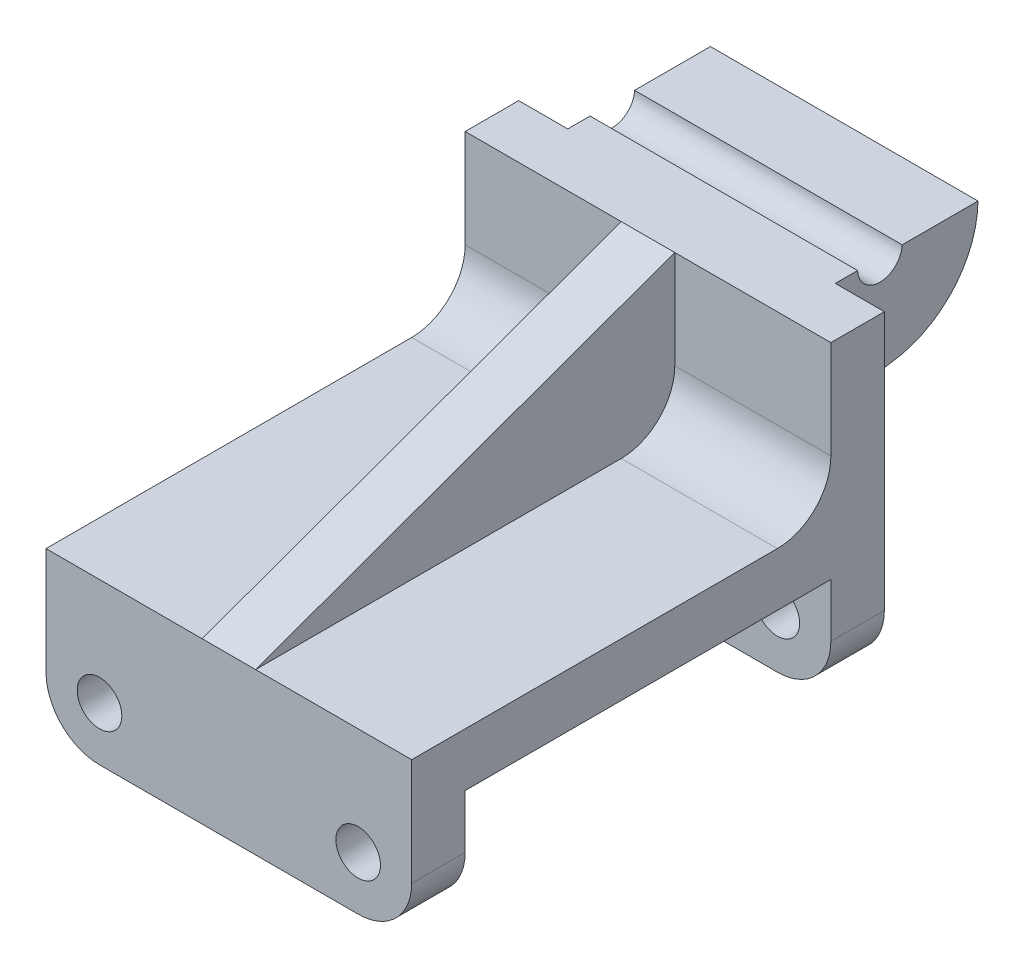
ISO-10303-21;
HEADER;
FILE_DESCRIPTION(('STEP AP214'),'2;1');
FILE_NAME('part.step','',(''),(''),'','','');
FILE_SCHEMA(('AUTOMOTIVE_DESIGN { 1 0 10303 214 1 1 1 1 }'));
ENDSEC;
DATA;
#1=APPLICATION_CONTEXT('core data for automotive mechanical design processes');
#2=APPLICATION_PROTOCOL_DEFINITION('international standard','automotive_design',2000,#1);
#3=PRODUCT_CONTEXT('',#1,'mechanical');
#4=PRODUCT('Part','Part','',(#3));
#5=PRODUCT_RELATED_PRODUCT_CATEGORY('part','',(#4));
#6=PRODUCT_DEFINITION_FORMATION('','',#4);
#7=PRODUCT_DEFINITION_CONTEXT('part definition',#1,'design');
#8=PRODUCT_DEFINITION('design','',#6,#7);
#9=PRODUCT_DEFINITION_SHAPE('','',#8);
#10=(LENGTH_UNIT() NAMED_UNIT(*) SI_UNIT(.MILLI.,.METRE.));
#11=(NAMED_UNIT(*) PLANE_ANGLE_UNIT() SI_UNIT($,.RADIAN.));
#12=(NAMED_UNIT(*) SI_UNIT($,.STERADIAN.) SOLID_ANGLE_UNIT());
#13=UNCERTAINTY_MEASURE_WITH_UNIT(LENGTH_MEASURE(1.E-05),#10,'distance_accuracy_value','');
#14=(GEOMETRIC_REPRESENTATION_CONTEXT(3) GLOBAL_UNCERTAINTY_ASSIGNED_CONTEXT((#13)) GLOBAL_UNIT_ASSIGNED_CONTEXT((#10,
#11,#12)) REPRESENTATION_CONTEXT('',''));
#15=CARTESIAN_POINT('',(0.,0.,0.));
#16=DIRECTION('',(0.,0.,1.));
#17=DIRECTION('',(1.,0.,0.));
#18=AXIS2_PLACEMENT_3D('',#15,#16,#17);
#19=CARTESIAN_POINT('',(82.,70.,-94.));
#20=DIRECTION('',(0.,0.,-1.));
#21=DIRECTION('',(-1.,0.,0.));
#22=AXIS2_PLACEMENT_3D('',#19,#20,#21);
#23=PLANE('',#22);
#24=DIRECTION('',(0.,-1.,0.));
#25=VECTOR('',#24,1.);
#26=CARTESIAN_POINT('',(0.,70.,-94.));
#27=LINE('',#26,#25);
#28=CARTESIAN_POINT('',(0.,70.,-94.));
#29=VERTEX_POINT('',#28);
#30=CARTESIAN_POINT('',(0.,48.,-94.));
#31=VERTEX_POINT('',#30);
#32=EDGE_CURVE('E315',#29,#31,#27,.T.);
#33=ORIENTED_EDGE('',*,*,#32,.T.);
#34=DIRECTION('',(-1.,0.,0.));
#35=VECTOR('',#34,1.);
#36=CARTESIAN_POINT('',(35.,48.,-94.));
#37=LINE('',#36,#35);
#38=CARTESIAN_POINT('',(35.,48.,-94.));
#39=VERTEX_POINT('',#38);
#40=EDGE_CURVE('E298',#31,#39,#37,.F.);
#41=ORIENTED_EDGE('',*,*,#40,.T.);
#42=DIRECTION('',(0.,-1.,0.));
#43=VECTOR('',#42,1.);
#44=CARTESIAN_POINT('',(35.,70.,-94.));
#45=LINE('',#44,#43);
#46=CARTESIAN_POINT('',(35.,70.,-94.));
#47=VERTEX_POINT('',#46);
#48=EDGE_CURVE('E335',#47,#39,#45,.T.);
#49=ORIENTED_EDGE('',*,*,#48,.F.);
#50=DIRECTION('',(-1.,0.,0.));
#51=VECTOR('',#50,1.);
#52=CARTESIAN_POINT('',(82.,70.,-94.));
#53=LINE('',#52,#51);
#54=EDGE_CURVE('E321',#47,#29,#53,.T.);
#55=ORIENTED_EDGE('',*,*,#54,.T.);
#56=EDGE_LOOP('',(#33,#41,#49,#55));
#57=FACE_BOUND('',#56,.T.);
#58=ADVANCED_FACE('F39',(#57),#23,.F.);
#59=CARTESIAN_POINT('',(82.,36.,-94.));
#60=DIRECTION('',(0.,-1.,0.));
#61=DIRECTION('',(0.,0.,-1.));
#62=AXIS2_PLACEMENT_3D('',#59,#60,#61);
#63=PLANE('',#62);
#64=DIRECTION('',(0.,0.,1.));
#65=VECTOR('',#64,1.);
#66=CARTESIAN_POINT('',(35.,36.,-94.));
#67=LINE('',#66,#65);
#68=CARTESIAN_POINT('',(35.,36.,-82.));
#69=VERTEX_POINT('',#68);
#70=CARTESIAN_POINT('',(35.,36.,0.));
#71=VERTEX_POINT('',#70);
#72=EDGE_CURVE('E289',#69,#71,#67,.T.);
#73=ORIENTED_EDGE('',*,*,#72,.F.);
#74=DIRECTION('',(-1.,0.,0.));
#75=VECTOR('',#74,1.);
#76=CARTESIAN_POINT('',(0.,36.,-82.));
#77=LINE('',#76,#75);
#78=CARTESIAN_POINT('',(0.,36.,-82.));
#79=VERTEX_POINT('',#78);
#80=EDGE_CURVE('E291',#69,#79,#77,.T.);
#81=ORIENTED_EDGE('',*,*,#80,.T.);
#82=DIRECTION('',(0.,0.,1.));
#83=VECTOR('',#82,1.);
#84=CARTESIAN_POINT('',(0.,36.,-94.));
#85=LINE('',#84,#83);
#86=CARTESIAN_POINT('',(0.,36.,0.));
#87=VERTEX_POINT('',#86);
#88=EDGE_CURVE('E314',#79,#87,#85,.T.);
#89=ORIENTED_EDGE('',*,*,#88,.T.);
#90=DIRECTION('',(-1.,0.,0.));
#91=VECTOR('',#90,1.);
#92=CARTESIAN_POINT('',(82.,36.,0.));
#93=LINE('',#92,#91);
#94=EDGE_CURVE('E340',#71,#87,#93,.T.);
#95=ORIENTED_EDGE('',*,*,#94,.F.);
#96=EDGE_LOOP('',(#73,#81,#89,#95));
#97=FACE_BOUND('',#96,.T.);
#98=ADVANCED_FACE('F333',(#97),#63,.F.);
#99=CARTESIAN_POINT('',(82.,36.,0.));
#100=DIRECTION('',(0.,0.,-1.));
#101=DIRECTION('',(0.,1.,0.));
#102=AXIS2_PLACEMENT_3D('',#99,#100,#101);
#103=PLANE('',#102);
#104=CARTESIAN_POINT('',(70.,12.,0.));
#105=DIRECTION('',(0.,0.,1.));
#106=DIRECTION('',(1.,0.,0.));
#107=AXIS2_PLACEMENT_3D('',#104,#105,#106);
#108=CIRCLE('',#107,5.);
#109=CARTESIAN_POINT('',(75.,12.,0.));
#110=VERTEX_POINT('',#109);
#111=EDGE_CURVE('E362',#110,#110,#108,.T.);
#112=ORIENTED_EDGE('',*,*,#111,.F.);
#113=EDGE_LOOP('',(#112));
#114=FACE_BOUND('',#113,.T.);
#115=CARTESIAN_POINT('',(82.,36.,0.));
#116=VERTEX_POINT('',#115);
#117=CARTESIAN_POINT('',(47.,36.,0.));
#118=VERTEX_POINT('',#117);
#119=EDGE_CURVE('E343',#116,#118,#93,.T.);
#120=ORIENTED_EDGE('',*,*,#119,.T.);
#121=EDGE_CURVE('E342',#118,#71,#93,.T.);
#122=ORIENTED_EDGE('',*,*,#121,.T.);
#123=ORIENTED_EDGE('',*,*,#94,.T.);
#124=DIRECTION('',(0.,-1.,0.));
#125=VECTOR('',#124,1.);
#126=CARTESIAN_POINT('',(0.,36.,0.));
#127=LINE('',#126,#125);
#128=CARTESIAN_POINT('',(0.,12.,0.));
#129=VERTEX_POINT('',#128);
#130=EDGE_CURVE('E387',#87,#129,#127,.T.);
#131=ORIENTED_EDGE('',*,*,#130,.T.);
#132=CARTESIAN_POINT('',(12.,12.,0.));
#133=DIRECTION('',(0.,0.,-1.));
#134=DIRECTION('',(0.,1.,0.));
#135=AXIS2_PLACEMENT_3D('',#132,#133,#134);
#136=CIRCLE('',#135,12.);
#137=CARTESIAN_POINT('',(12.,0.,0.));
#138=VERTEX_POINT('',#137);
#139=EDGE_CURVE('E287',#129,#138,#136,.F.);
#140=ORIENTED_EDGE('',*,*,#139,.T.);
#141=DIRECTION('',(-1.,0.,0.));
#142=VECTOR('',#141,1.);
#143=CARTESIAN_POINT('',(82.,0.,0.));
#144=LINE('',#143,#142);
#145=CARTESIAN_POINT('',(70.,0.,0.));
#146=VERTEX_POINT('',#145);
#147=EDGE_CURVE('E249',#146,#138,#144,.T.);
#148=ORIENTED_EDGE('',*,*,#147,.F.);
#149=CARTESIAN_POINT('',(70.,12.,0.));
#150=DIRECTION('',(0.,0.,-1.));
#151=DIRECTION('',(0.,1.,0.));
#152=AXIS2_PLACEMENT_3D('',#149,#150,#151);
#153=CIRCLE('',#152,12.);
#154=CARTESIAN_POINT('',(82.,12.,0.));
#155=VERTEX_POINT('',#154);
#156=EDGE_CURVE('E284',#146,#155,#153,.F.);
#157=ORIENTED_EDGE('',*,*,#156,.T.);
#158=DIRECTION('',(0.,-1.,0.));
#159=VECTOR('',#158,1.);
#160=CARTESIAN_POINT('',(82.,36.,0.));
#161=LINE('',#160,#159);
#162=EDGE_CURVE('E390',#116,#155,#161,.T.);
#163=ORIENTED_EDGE('',*,*,#162,.F.);
#164=EDGE_LOOP('',(#120,#122,#123,#131,#140,#148,#157,#163));
#165=FACE_BOUND('',#164,.T.);
#166=CARTESIAN_POINT('',(12.,12.,0.));
#167=DIRECTION('',(0.,0.,1.));
#168=DIRECTION('',(1.,0.,0.));
#169=AXIS2_PLACEMENT_3D('',#166,#167,#168);
#170=CIRCLE('',#169,5.);
#171=CARTESIAN_POINT('',(17.,12.,0.));
#172=VERTEX_POINT('',#171);
#173=EDGE_CURVE('E370',#172,#172,#170,.T.);
#174=ORIENTED_EDGE('',*,*,#173,.F.);
#175=EDGE_LOOP('',(#174));
#176=FACE_BOUND('',#175,.T.);
#177=ADVANCED_FACE('F419',(#114,#165,#176),#103,.F.);
#178=CARTESIAN_POINT('',(82.,0.,0.));
#179=DIRECTION('',(0.,1.,0.));
#180=DIRECTION('',(0.,0.,1.));
#181=AXIS2_PLACEMENT_3D('',#178,#179,#180);
#182=PLANE('',#181);
#183=ORIENTED_EDGE('',*,*,#147,.T.);
#184=DIRECTION('',(0.,0.,-1.));
#185=VECTOR('',#184,1.);
#186=CARTESIAN_POINT('',(12.,0.,0.));
#187=LINE('',#186,#185);
#188=CARTESIAN_POINT('',(12.,0.,-12.));
#189=VERTEX_POINT('',#188);
#190=EDGE_CURVE('E280',#138,#189,#187,.T.);
#191=ORIENTED_EDGE('',*,*,#190,.T.);
#192=DIRECTION('',(-1.,0.,0.));
#193=VECTOR('',#192,1.);
#194=CARTESIAN_POINT('',(82.,0.,-12.));
#195=LINE('',#194,#193);
#196=CARTESIAN_POINT('',(70.,0.,-12.));
#197=VERTEX_POINT('',#196);
#198=EDGE_CURVE('E250',#197,#189,#195,.T.);
#199=ORIENTED_EDGE('',*,*,#198,.F.);
#200=DIRECTION('',(0.,0.,-1.));
#201=VECTOR('',#200,1.);
#202=CARTESIAN_POINT('',(70.,0.,0.));
#203=LINE('',#202,#201);
#204=EDGE_CURVE('E274',#197,#146,#203,.F.);
#205=ORIENTED_EDGE('',*,*,#204,.T.);
#206=EDGE_LOOP('',(#183,#191,#199,#205));
#207=FACE_BOUND('',#206,.T.);
#208=ADVANCED_FACE('F421',(#207),#182,.F.);
#209=CARTESIAN_POINT('',(82.,0.,-12.));
#210=DIRECTION('',(0.,0.,1.));
#211=DIRECTION('',(0.,-1.,0.));
#212=AXIS2_PLACEMENT_3D('',#209,#210,#211);
#213=PLANE('',#212);
#214=CARTESIAN_POINT('',(70.,12.,-12.));
#215=DIRECTION('',(0.,0.,1.));
#216=DIRECTION('',(0.,-1.,0.));
#217=AXIS2_PLACEMENT_3D('',#214,#215,#216);
#218=CIRCLE('',#217,5.);
#219=CARTESIAN_POINT('',(70.,7.,-12.));
#220=VERTEX_POINT('',#219);
#221=EDGE_CURVE('E380',#220,#220,#218,.T.);
#222=ORIENTED_EDGE('',*,*,#221,.T.);
#223=EDGE_LOOP('',(#222));
#224=FACE_BOUND('',#223,.T.);
#225=ORIENTED_EDGE('',*,*,#198,.T.);
#226=CARTESIAN_POINT('',(12.,12.,-12.));
#227=DIRECTION('',(0.,0.,1.));
#228=DIRECTION('',(0.,-1.,0.));
#229=AXIS2_PLACEMENT_3D('',#226,#227,#228);
#230=CIRCLE('',#229,12.);
#231=CARTESIAN_POINT('',(0.,12.,-12.));
#232=VERTEX_POINT('',#231);
#233=EDGE_CURVE('E285',#189,#232,#230,.F.);
#234=ORIENTED_EDGE('',*,*,#233,.T.);
#235=DIRECTION('',(0.,1.,0.));
#236=VECTOR('',#235,1.);
#237=CARTESIAN_POINT('',(0.,0.,-12.));
#238=LINE('',#237,#236);
#239=CARTESIAN_POINT('',(0.,24.,-12.));
#240=VERTEX_POINT('',#239);
#241=EDGE_CURVE('E404',#232,#240,#238,.T.);
#242=ORIENTED_EDGE('',*,*,#241,.T.);
#243=DIRECTION('',(-1.,0.,0.));
#244=VECTOR('',#243,1.);
#245=CARTESIAN_POINT('',(82.,24.,-12.));
#246=LINE('',#245,#244);
#247=CARTESIAN_POINT('',(82.,24.,-12.));
#248=VERTEX_POINT('',#247);
#249=EDGE_CURVE('E242',#248,#240,#246,.T.);
#250=ORIENTED_EDGE('',*,*,#249,.F.);
#251=DIRECTION('',(0.,1.,0.));
#252=VECTOR('',#251,1.);
#253=CARTESIAN_POINT('',(82.,0.,-12.));
#254=LINE('',#253,#252);
#255=CARTESIAN_POINT('',(82.,12.,-12.));
#256=VERTEX_POINT('',#255);
#257=EDGE_CURVE('E388',#256,#248,#254,.T.);
#258=ORIENTED_EDGE('',*,*,#257,.F.);
#259=CARTESIAN_POINT('',(70.,12.,-12.));
#260=DIRECTION('',(0.,0.,1.));
#261=DIRECTION('',(0.,-1.,0.));
#262=AXIS2_PLACEMENT_3D('',#259,#260,#261);
#263=CIRCLE('',#262,12.);
#264=EDGE_CURVE('E278',#256,#197,#263,.F.);
#265=ORIENTED_EDGE('',*,*,#264,.T.);
#266=EDGE_LOOP('',(#225,#234,#242,#250,#258,#265));
#267=FACE_BOUND('',#266,.T.);
#268=CARTESIAN_POINT('',(12.,12.,-12.));
#269=DIRECTION('',(0.,0.,1.));
#270=DIRECTION('',(0.,-1.,0.));
#271=AXIS2_PLACEMENT_3D('',#268,#269,#270);
#272=CIRCLE('',#271,5.);
#273=CARTESIAN_POINT('',(12.,7.,-12.));
#274=VERTEX_POINT('',#273);
#275=EDGE_CURVE('E382',#274,#274,#272,.T.);
#276=ORIENTED_EDGE('',*,*,#275,.T.);
#277=EDGE_LOOP('',(#276));
#278=FACE_BOUND('',#277,.T.);
#279=ADVANCED_FACE('F436',(#224,#267,#278),#213,.F.);
#280=CARTESIAN_POINT('',(82.,24.,-12.));
#281=DIRECTION('',(0.,1.,0.));
#282=DIRECTION('',(0.,0.,1.));
#283=AXIS2_PLACEMENT_3D('',#280,#281,#282);
#284=PLANE('',#283);
#285=ORIENTED_EDGE('',*,*,#249,.T.);
#286=DIRECTION('',(0.,0.,-1.));
#287=VECTOR('',#286,1.);
#288=CARTESIAN_POINT('',(0.,24.,-12.));
#289=LINE('',#288,#287);
#290=CARTESIAN_POINT('',(0.,24.,-94.));
#291=VERTEX_POINT('',#290);
#292=EDGE_CURVE('E410',#240,#291,#289,.T.);
#293=ORIENTED_EDGE('',*,*,#292,.T.);
#294=DIRECTION('',(-1.,0.,0.));
#295=VECTOR('',#294,1.);
#296=CARTESIAN_POINT('',(82.,24.,-94.));
#297=LINE('',#296,#295);
#298=CARTESIAN_POINT('',(82.,24.,-94.));
#299=VERTEX_POINT('',#298);
#300=EDGE_CURVE('E241',#299,#291,#297,.T.);
#301=ORIENTED_EDGE('',*,*,#300,.F.);
#302=DIRECTION('',(0.,0.,-1.));
#303=VECTOR('',#302,1.);
#304=CARTESIAN_POINT('',(82.,24.,-12.));
#305=LINE('',#304,#303);
#306=EDGE_CURVE('E395',#248,#299,#305,.T.);
#307=ORIENTED_EDGE('',*,*,#306,.F.);
#308=EDGE_LOOP('',(#285,#293,#301,#307));
#309=FACE_BOUND('',#308,.T.);
#310=ADVANCED_FACE('F437',(#309),#284,.F.);
#311=CARTESIAN_POINT('',(82.,24.,-94.));
#312=DIRECTION('',(0.,0.,-1.));
#313=DIRECTION('',(0.,1.,0.));
#314=AXIS2_PLACEMENT_3D('',#311,#312,#313);
#315=PLANE('',#314);
#316=CARTESIAN_POINT('',(70.,12.,-94.));
#317=DIRECTION('',(0.,0.,-1.));
#318=DIRECTION('',(0.,1.,0.));
#319=AXIS2_PLACEMENT_3D('',#316,#317,#318);
#320=CIRCLE('',#319,5.);
#321=CARTESIAN_POINT('',(70.,17.,-94.));
#322=VERTEX_POINT('',#321);
#323=EDGE_CURVE('E368',#322,#322,#320,.T.);
#324=ORIENTED_EDGE('',*,*,#323,.T.);
#325=EDGE_LOOP('',(#324));
#326=FACE_BOUND('',#325,.T.);
#327=ORIENTED_EDGE('',*,*,#300,.T.);
#328=DIRECTION('',(0.,-1.,0.));
#329=VECTOR('',#328,1.);
#330=CARTESIAN_POINT('',(0.,24.,-94.));
#331=LINE('',#330,#329);
#332=CARTESIAN_POINT('',(0.,12.,-94.));
#333=VERTEX_POINT('',#332);
#334=EDGE_CURVE('E407',#291,#333,#331,.T.);
#335=ORIENTED_EDGE('',*,*,#334,.T.);
#336=CARTESIAN_POINT('',(12.,12.,-94.));
#337=DIRECTION('',(0.,0.,-1.));
#338=DIRECTION('',(0.,1.,0.));
#339=AXIS2_PLACEMENT_3D('',#336,#337,#338);
#340=CIRCLE('',#339,12.);
#341=CARTESIAN_POINT('',(12.,0.,-94.));
#342=VERTEX_POINT('',#341);
#343=EDGE_CURVE('E266',#333,#342,#340,.F.);
#344=ORIENTED_EDGE('',*,*,#343,.T.);
#345=DIRECTION('',(-1.,0.,0.));
#346=VECTOR('',#345,1.);
#347=CARTESIAN_POINT('',(82.,0.,-94.));
#348=LINE('',#347,#346);
#349=CARTESIAN_POINT('',(70.,0.,-94.));
#350=VERTEX_POINT('',#349);
#351=EDGE_CURVE('E237',#350,#342,#348,.T.);
#352=ORIENTED_EDGE('',*,*,#351,.F.);
#353=CARTESIAN_POINT('',(70.,12.,-94.));
#354=DIRECTION('',(0.,0.,-1.));
#355=DIRECTION('',(0.,1.,0.));
#356=AXIS2_PLACEMENT_3D('',#353,#354,#355);
#357=CIRCLE('',#356,12.);
#358=CARTESIAN_POINT('',(82.,12.,-94.));
#359=VERTEX_POINT('',#358);
#360=EDGE_CURVE('E267',#350,#359,#357,.F.);
#361=ORIENTED_EDGE('',*,*,#360,.T.);
#362=DIRECTION('',(0.,-1.,0.));
#363=VECTOR('',#362,1.);
#364=CARTESIAN_POINT('',(82.,24.,-94.));
#365=LINE('',#364,#363);
#366=EDGE_CURVE('E394',#299,#359,#365,.T.);
#367=ORIENTED_EDGE('',*,*,#366,.F.);
#368=EDGE_LOOP('',(#327,#335,#344,#352,#361,#367));
#369=FACE_BOUND('',#368,.T.);
#370=CARTESIAN_POINT('',(12.,12.,-94.));
#371=DIRECTION('',(0.,0.,-1.));
#372=DIRECTION('',(0.,1.,0.));
#373=AXIS2_PLACEMENT_3D('',#370,#371,#372);
#374=CIRCLE('',#373,5.);
#375=CARTESIAN_POINT('',(12.,17.,-94.));
#376=VERTEX_POINT('',#375);
#377=EDGE_CURVE('E379',#376,#376,#374,.T.);
#378=ORIENTED_EDGE('',*,*,#377,.T.);
#379=EDGE_LOOP('',(#378));
#380=FACE_BOUND('',#379,.T.);
#381=ADVANCED_FACE('F443',(#326,#369,#380),#315,.F.);
#382=CARTESIAN_POINT('',(82.,0.,-94.));
#383=DIRECTION('',(0.,1.,0.));
#384=DIRECTION('',(0.,0.,1.));
#385=AXIS2_PLACEMENT_3D('',#382,#383,#384);
#386=PLANE('',#385);
#387=ORIENTED_EDGE('',*,*,#351,.T.);
#388=DIRECTION('',(0.,0.,-1.));
#389=VECTOR('',#388,1.);
#390=CARTESIAN_POINT('',(12.,0.,-94.));
#391=LINE('',#390,#389);
#392=CARTESIAN_POINT('',(12.,0.,-106.));
#393=VERTEX_POINT('',#392);
#394=EDGE_CURVE('E261',#342,#393,#391,.T.);
#395=ORIENTED_EDGE('',*,*,#394,.T.);
#396=DIRECTION('',(-1.,0.,0.));
#397=VECTOR('',#396,1.);
#398=CARTESIAN_POINT('',(82.,0.,-106.));
#399=LINE('',#398,#397);
#400=CARTESIAN_POINT('',(70.,0.,-106.));
#401=VERTEX_POINT('',#400);
#402=EDGE_CURVE('E233',#401,#393,#399,.T.);
#403=ORIENTED_EDGE('',*,*,#402,.F.);
#404=DIRECTION('',(0.,0.,-1.));
#405=VECTOR('',#404,1.);
#406=CARTESIAN_POINT('',(70.,0.,-94.));
#407=LINE('',#406,#405);
#408=EDGE_CURVE('E262',#401,#350,#407,.F.);
#409=ORIENTED_EDGE('',*,*,#408,.T.);
#410=EDGE_LOOP('',(#387,#395,#403,#409));
#411=FACE_BOUND('',#410,.T.);
#412=ADVANCED_FACE('F510',(#411),#386,.F.);
#413=CARTESIAN_POINT('',(82.,0.,-106.));
#414=DIRECTION('',(0.,0.,1.));
#415=DIRECTION('',(0.,-1.,0.));
#416=AXIS2_PLACEMENT_3D('',#413,#414,#415);
#417=PLANE('',#416);
#418=CARTESIAN_POINT('',(70.,12.,-106.));
#419=DIRECTION('',(0.,0.,1.));
#420=DIRECTION('',(1.,0.,0.));
#421=AXIS2_PLACEMENT_3D('',#418,#419,#420);
#422=CIRCLE('',#421,5.);
#423=CARTESIAN_POINT('',(75.,12.,-106.));
#424=VERTEX_POINT('',#423);
#425=EDGE_CURVE('E367',#424,#424,#422,.T.);
#426=ORIENTED_EDGE('',*,*,#425,.T.);
#427=EDGE_LOOP('',(#426));
#428=FACE_BOUND('',#427,.T.);
#429=DIRECTION('',(-1.,0.,0.));
#430=VECTOR('',#429,1.);
#431=CARTESIAN_POINT('',(71.,34.4490250994304,-106.));
#432=LINE('',#431,#430);
#433=CARTESIAN_POINT('',(71.,34.4490250994304,-106.));
#434=VERTEX_POINT('',#433);
#435=CARTESIAN_POINT('',(11.,34.4490250994304,-106.));
#436=VERTEX_POINT('',#435);
#437=EDGE_CURVE('E230',#434,#436,#432,.T.);
#438=ORIENTED_EDGE('',*,*,#437,.F.);
#439=DIRECTION('',(0.,-1.,0.));
#440=VECTOR('',#439,1.);
#441=CARTESIAN_POINT('',(71.,34.4490250994304,-106.));
#442=LINE('',#441,#440);
#443=CARTESIAN_POINT('',(71.,70.,-106.));
#444=VERTEX_POINT('',#443);
#445=EDGE_CURVE('E209',#444,#434,#442,.T.);
#446=ORIENTED_EDGE('',*,*,#445,.F.);
#447=DIRECTION('',(-1.,0.,0.));
#448=VECTOR('',#447,1.);
#449=CARTESIAN_POINT('',(82.,70.,-106.));
#450=LINE('',#449,#448);
#451=CARTESIAN_POINT('',(82.,70.,-106.));
#452=VERTEX_POINT('',#451);
#453=EDGE_CURVE('E221',#452,#444,#450,.T.);
#454=ORIENTED_EDGE('',*,*,#453,.F.);
#455=DIRECTION('',(0.,1.,0.));
#456=VECTOR('',#455,1.);
#457=CARTESIAN_POINT('',(82.,0.,-106.));
#458=LINE('',#457,#456);
#459=CARTESIAN_POINT('',(82.,12.,-106.));
#460=VERTEX_POINT('',#459);
#461=EDGE_CURVE('E400',#460,#452,#458,.T.);
#462=ORIENTED_EDGE('',*,*,#461,.F.);
#463=CARTESIAN_POINT('',(70.,12.,-106.));
#464=DIRECTION('',(0.,0.,1.));
#465=DIRECTION('',(0.,-1.,0.));
#466=AXIS2_PLACEMENT_3D('',#463,#464,#465);
#467=CIRCLE('',#466,12.);
#468=EDGE_CURVE('E259',#460,#401,#467,.F.);
#469=ORIENTED_EDGE('',*,*,#468,.T.);
#470=ORIENTED_EDGE('',*,*,#402,.T.);
#471=CARTESIAN_POINT('',(12.,12.,-106.));
#472=DIRECTION('',(0.,0.,1.));
#473=DIRECTION('',(0.,-1.,0.));
#474=AXIS2_PLACEMENT_3D('',#471,#472,#473);
#475=CIRCLE('',#474,12.);
#476=CARTESIAN_POINT('',(0.,12.,-106.));
#477=VERTEX_POINT('',#476);
#478=EDGE_CURVE('E260',#393,#477,#475,.F.);
#479=ORIENTED_EDGE('',*,*,#478,.T.);
#480=DIRECTION('',(0.,1.,0.));
#481=VECTOR('',#480,1.);
#482=CARTESIAN_POINT('',(0.,0.,-106.));
#483=LINE('',#482,#481);
#484=CARTESIAN_POINT('',(0.,70.,-106.));
#485=VERTEX_POINT('',#484);
#486=EDGE_CURVE('E413',#477,#485,#483,.T.);
#487=ORIENTED_EDGE('',*,*,#486,.T.);
#488=CARTESIAN_POINT('',(11.,70.,-106.));
#489=VERTEX_POINT('',#488);
#490=EDGE_CURVE('E234',#489,#485,#450,.T.);
#491=ORIENTED_EDGE('',*,*,#490,.F.);
#492=DIRECTION('',(0.,-1.,0.));
#493=VECTOR('',#492,1.);
#494=CARTESIAN_POINT('',(11.,34.4490250994304,-106.));
#495=LINE('',#494,#493);
#496=EDGE_CURVE('E513',#489,#436,#495,.T.);
#497=ORIENTED_EDGE('',*,*,#496,.T.);
#498=EDGE_LOOP('',(#438,#446,#454,#462,#469,#470,#479,#487,#491,#497));
#499=FACE_BOUND('',#498,.T.);
#500=CARTESIAN_POINT('',(12.,12.,-106.));
#501=DIRECTION('',(0.,0.,1.));
#502=DIRECTION('',(1.,0.,0.));
#503=AXIS2_PLACEMENT_3D('',#500,#501,#502);
#504=CIRCLE('',#503,5.);
#505=CARTESIAN_POINT('',(17.,12.,-106.));
#506=VERTEX_POINT('',#505);
#507=EDGE_CURVE('E361',#506,#506,#504,.T.);
#508=ORIENTED_EDGE('',*,*,#507,.T.);
#509=EDGE_LOOP('',(#508));
#510=FACE_BOUND('',#509,.T.);
#511=ADVANCED_FACE('F222',(#428,#499,#510),#417,.F.);
#512=CARTESIAN_POINT('',(82.,70.,-106.));
#513=DIRECTION('',(0.,-1.,0.));
#514=DIRECTION('',(0.,0.,-1.));
#515=AXIS2_PLACEMENT_3D('',#512,#513,#514);
#516=PLANE('',#515);
#517=ORIENTED_EDGE('',*,*,#453,.T.);
#518=DIRECTION('',(0.,0.,1.));
#519=VECTOR('',#518,1.);
#520=CARTESIAN_POINT('',(71.,70.,-106.));
#521=LINE('',#520,#519);
#522=CARTESIAN_POINT('',(71.,70.,-111.005115313737));
#523=VERTEX_POINT('',#522);
#524=EDGE_CURVE('E210',#523,#444,#521,.T.);
#525=ORIENTED_EDGE('',*,*,#524,.F.);
#526=DIRECTION('',(-1.,0.,0.));
#527=VECTOR('',#526,1.);
#528=CARTESIAN_POINT('',(71.,70.,-111.005115313737));
#529=LINE('',#528,#527);
#530=CARTESIAN_POINT('',(11.,70.,-111.005115313737));
#531=VERTEX_POINT('',#530);
#532=EDGE_CURVE('E530',#523,#531,#529,.T.);
#533=ORIENTED_EDGE('',*,*,#532,.T.);
#534=DIRECTION('',(0.,0.,1.));
#535=VECTOR('',#534,1.);
#536=CARTESIAN_POINT('',(11.,70.,-106.));
#537=LINE('',#536,#535);
#538=EDGE_CURVE('E53',#531,#489,#537,.T.);
#539=ORIENTED_EDGE('',*,*,#538,.T.);
#540=ORIENTED_EDGE('',*,*,#490,.T.);
#541=DIRECTION('',(0.,0.,1.));
#542=VECTOR('',#541,1.);
#543=CARTESIAN_POINT('',(0.,70.,-106.));
#544=LINE('',#543,#542);
#545=EDGE_CURVE('E323',#485,#29,#544,.T.);
#546=ORIENTED_EDGE('',*,*,#545,.T.);
#547=ORIENTED_EDGE('',*,*,#54,.F.);
#548=DIRECTION('',(1.,0.,0.));
#549=VECTOR('',#548,1.);
#550=CARTESIAN_POINT('',(82.,70.,-94.));
#551=LINE('',#550,#549);
#552=CARTESIAN_POINT('',(47.,70.,-94.));
#553=VERTEX_POINT('',#552);
#554=EDGE_CURVE('E353',#47,#553,#551,.T.);
#555=ORIENTED_EDGE('',*,*,#554,.T.);
#556=CARTESIAN_POINT('',(82.,70.,-94.));
#557=VERTEX_POINT('',#556);
#558=EDGE_CURVE('E236',#557,#553,#53,.T.);
#559=ORIENTED_EDGE('',*,*,#558,.F.);
#560=DIRECTION('',(0.,0.,1.));
#561=VECTOR('',#560,1.);
#562=CARTESIAN_POINT('',(82.,70.,-106.));
#563=LINE('',#562,#561);
#564=EDGE_CURVE('E235',#452,#557,#563,.T.);
#565=ORIENTED_EDGE('',*,*,#564,.F.);
#566=EDGE_LOOP('',(#517,#525,#533,#539,#540,#546,#547,#555,#559,#565));
#567=FACE_BOUND('',#566,.T.);
#568=ADVANCED_FACE('F227',(#567),#516,.F.);
#569=DIRECTION('',(0.,-1.,0.));
#570=VECTOR('',#569,1.);
#571=CARTESIAN_POINT('',(47.,70.,-94.));
#572=LINE('',#571,#570);
#573=CARTESIAN_POINT('',(47.,48.,-94.));
#574=VERTEX_POINT('',#573);
#575=EDGE_CURVE('E359',#553,#574,#572,.T.);
#576=ORIENTED_EDGE('',*,*,#575,.T.);
#577=DIRECTION('',(-1.,0.,0.));
#578=VECTOR('',#577,1.);
#579=CARTESIAN_POINT('',(82.,48.,-94.));
#580=LINE('',#579,#578);
#581=CARTESIAN_POINT('',(82.,48.,-94.));
#582=VERTEX_POINT('',#581);
#583=EDGE_CURVE('E65',#574,#582,#580,.F.);
#584=ORIENTED_EDGE('',*,*,#583,.T.);
#585=DIRECTION('',(0.,-1.,0.));
#586=VECTOR('',#585,1.);
#587=CARTESIAN_POINT('',(82.,70.,-94.));
#588=LINE('',#587,#586);
#589=EDGE_CURVE('E396',#557,#582,#588,.T.);
#590=ORIENTED_EDGE('',*,*,#589,.F.);
#591=ORIENTED_EDGE('',*,*,#558,.T.);
#592=EDGE_LOOP('',(#576,#584,#590,#591));
#593=FACE_BOUND('',#592,.T.);
#594=ADVANCED_FACE('F453',(#593),#23,.F.);
#595=DIRECTION('',(0.,0.,1.));
#596=VECTOR('',#595,1.);
#597=CARTESIAN_POINT('',(82.,36.,-94.));
#598=LINE('',#597,#596);
#599=CARTESIAN_POINT('',(82.,36.,-82.));
#600=VERTEX_POINT('',#599);
#601=EDGE_CURVE('E345',#600,#116,#598,.T.);
#602=ORIENTED_EDGE('',*,*,#601,.F.);
#603=DIRECTION('',(-1.,0.,0.));
#604=VECTOR('',#603,1.);
#605=CARTESIAN_POINT('',(47.,36.,-82.));
#606=LINE('',#605,#604);
#607=CARTESIAN_POINT('',(47.,36.,-82.));
#608=VERTEX_POINT('',#607);
#609=EDGE_CURVE('E297',#600,#608,#606,.T.);
#610=ORIENTED_EDGE('',*,*,#609,.T.);
#611=DIRECTION('',(0.,0.,1.));
#612=VECTOR('',#611,1.);
#613=CARTESIAN_POINT('',(47.,36.,-94.));
#614=LINE('',#613,#612);
#615=EDGE_CURVE('E292',#608,#118,#614,.T.);
#616=ORIENTED_EDGE('',*,*,#615,.T.);
#617=ORIENTED_EDGE('',*,*,#119,.F.);
#618=EDGE_LOOP('',(#602,#610,#616,#617));
#619=FACE_BOUND('',#618,.T.);
#620=ADVANCED_FACE('F459',(#619),#63,.F.);
#621=CARTESIAN_POINT('',(82.,0.,0.));
#622=DIRECTION('',(1.,0.,0.));
#623=DIRECTION('',(0.,0.,-1.));
#624=AXIS2_PLACEMENT_3D('',#621,#622,#623);
#625=PLANE('',#624);
#626=ORIENTED_EDGE('',*,*,#366,.T.);
#627=DIRECTION('',(0.,0.,-1.));
#628=VECTOR('',#627,1.);
#629=CARTESIAN_POINT('',(82.,12.,-106.));
#630=LINE('',#629,#628);
#631=EDGE_CURVE('E255',#359,#460,#630,.T.);
#632=ORIENTED_EDGE('',*,*,#631,.T.);
#633=ORIENTED_EDGE('',*,*,#461,.T.);
#634=ORIENTED_EDGE('',*,*,#564,.T.);
#635=ORIENTED_EDGE('',*,*,#589,.T.);
#636=CARTESIAN_POINT('',(82.,48.,-82.));
#637=DIRECTION('',(1.,0.,0.));
#638=DIRECTION('',(0.,0.,-1.));
#639=AXIS2_PLACEMENT_3D('',#636,#637,#638);
#640=CIRCLE('',#639,12.);
#641=EDGE_CURVE('E11',#582,#600,#640,.F.);
#642=ORIENTED_EDGE('',*,*,#641,.T.);
#643=ORIENTED_EDGE('',*,*,#601,.T.);
#644=ORIENTED_EDGE('',*,*,#162,.T.);
#645=DIRECTION('',(0.,0.,-1.));
#646=VECTOR('',#645,1.);
#647=CARTESIAN_POINT('',(82.,12.,-12.));
#648=LINE('',#647,#646);
#649=EDGE_CURVE('E253',#155,#256,#648,.T.);
#650=ORIENTED_EDGE('',*,*,#649,.T.);
#651=ORIENTED_EDGE('',*,*,#257,.T.);
#652=ORIENTED_EDGE('',*,*,#306,.T.);
#653=EDGE_LOOP('',(#626,#632,#633,#634,#635,#642,#643,#644,#650,#651,#652));
#654=FACE_BOUND('',#653,.T.);
#655=ADVANCED_FACE('F462',(#654),#625,.T.);
#656=CARTESIAN_POINT('',(0.,0.,0.));
#657=DIRECTION('',(1.,0.,0.));
#658=DIRECTION('',(0.,0.,-1.));
#659=AXIS2_PLACEMENT_3D('',#656,#657,#658);
#660=PLANE('',#659);
#661=ORIENTED_EDGE('',*,*,#486,.F.);
#662=DIRECTION('',(0.,0.,-1.));
#663=VECTOR('',#662,1.);
#664=CARTESIAN_POINT('',(0.,12.,0.));
#665=LINE('',#664,#663);
#666=EDGE_CURVE('E272',#477,#333,#665,.F.);
#667=ORIENTED_EDGE('',*,*,#666,.T.);
#668=ORIENTED_EDGE('',*,*,#334,.F.);
#669=ORIENTED_EDGE('',*,*,#292,.F.);
#670=ORIENTED_EDGE('',*,*,#241,.F.);
#671=DIRECTION('',(0.,0.,-1.));
#672=VECTOR('',#671,1.);
#673=CARTESIAN_POINT('',(0.,12.,0.));
#674=LINE('',#673,#672);
#675=EDGE_CURVE('E271',#232,#129,#674,.F.);
#676=ORIENTED_EDGE('',*,*,#675,.T.);
#677=ORIENTED_EDGE('',*,*,#130,.F.);
#678=ORIENTED_EDGE('',*,*,#88,.F.);
#679=CARTESIAN_POINT('',(0.,48.,-82.));
#680=DIRECTION('',(1.,0.,0.));
#681=DIRECTION('',(0.,0.,-1.));
#682=AXIS2_PLACEMENT_3D('',#679,#680,#681);
#683=CIRCLE('',#682,12.);
#684=EDGE_CURVE('E50',#79,#31,#683,.T.);
#685=ORIENTED_EDGE('',*,*,#684,.T.);
#686=ORIENTED_EDGE('',*,*,#32,.F.);
#687=ORIENTED_EDGE('',*,*,#545,.F.);
#688=EDGE_LOOP('',(#661,#667,#668,#669,#670,#676,#677,#678,#685,#686,#687));
#689=FACE_BOUND('',#688,.T.);
#690=ADVANCED_FACE('F309',(#689),#660,.F.);
#691=CARTESIAN_POINT('',(70.,12.,0.));
#692=DIRECTION('',(0.,0.,1.));
#693=DIRECTION('',(1.,0.,0.));
#694=AXIS2_PLACEMENT_3D('',#691,#692,#693);
#695=CYLINDRICAL_SURFACE('',#694,12.);
#696=ORIENTED_EDGE('',*,*,#360,.F.);
#697=ORIENTED_EDGE('',*,*,#408,.F.);
#698=ORIENTED_EDGE('',*,*,#468,.F.);
#699=ORIENTED_EDGE('',*,*,#631,.F.);
#700=EDGE_LOOP('',(#696,#697,#698,#699));
#701=FACE_BOUND('',#700,.T.);
#702=ADVANCED_FACE('F505',(#701),#695,.T.);
#703=CARTESIAN_POINT('',(12.,12.,-94.));
#704=DIRECTION('',(0.,0.,-1.));
#705=DIRECTION('',(-1.,0.,0.));
#706=AXIS2_PLACEMENT_3D('',#703,#704,#705);
#707=CYLINDRICAL_SURFACE('',#706,12.);
#708=ORIENTED_EDGE('',*,*,#343,.F.);
#709=ORIENTED_EDGE('',*,*,#666,.F.);
#710=ORIENTED_EDGE('',*,*,#478,.F.);
#711=ORIENTED_EDGE('',*,*,#394,.F.);
#712=EDGE_LOOP('',(#708,#709,#710,#711));
#713=FACE_BOUND('',#712,.T.);
#714=ADVANCED_FACE('F515',(#713),#707,.T.);
#715=CARTESIAN_POINT('',(12.,12.,0.));
#716=DIRECTION('',(0.,0.,-1.));
#717=DIRECTION('',(-1.,0.,0.));
#718=AXIS2_PLACEMENT_3D('',#715,#716,#717);
#719=CYLINDRICAL_SURFACE('',#718,12.);
#720=ORIENTED_EDGE('',*,*,#139,.F.);
#721=ORIENTED_EDGE('',*,*,#675,.F.);
#722=ORIENTED_EDGE('',*,*,#233,.F.);
#723=ORIENTED_EDGE('',*,*,#190,.F.);
#724=EDGE_LOOP('',(#720,#721,#722,#723));
#725=FACE_BOUND('',#724,.T.);
#726=ADVANCED_FACE('F489',(#725),#719,.T.);
#727=CARTESIAN_POINT('',(70.,12.,0.));
#728=DIRECTION('',(0.,0.,1.));
#729=DIRECTION('',(1.,0.,0.));
#730=AXIS2_PLACEMENT_3D('',#727,#728,#729);
#731=CYLINDRICAL_SURFACE('',#730,12.);
#732=ORIENTED_EDGE('',*,*,#156,.F.);
#733=ORIENTED_EDGE('',*,*,#204,.F.);
#734=ORIENTED_EDGE('',*,*,#264,.F.);
#735=ORIENTED_EDGE('',*,*,#649,.F.);
#736=EDGE_LOOP('',(#732,#733,#734,#735));
#737=FACE_BOUND('',#736,.T.);
#738=ADVANCED_FACE('F485',(#737),#731,.T.);
#739=CARTESIAN_POINT('',(70.,12.,-106.));
#740=DIRECTION('',(0.,0.,1.));
#741=DIRECTION('',(1.,0.,0.));
#742=AXIS2_PLACEMENT_3D('',#739,#740,#741);
#743=CYLINDRICAL_SURFACE('',#742,5.);
#744=ORIENTED_EDGE('',*,*,#425,.F.);
#745=EDGE_LOOP('',(#744));
#746=FACE_BOUND('',#745,.T.);
#747=ORIENTED_EDGE('',*,*,#323,.F.);
#748=EDGE_LOOP('',(#747));
#749=FACE_BOUND('',#748,.T.);
#750=ADVANCED_FACE('F578',(#746,#749),#743,.F.);
#751=CARTESIAN_POINT('',(12.,12.,-106.));
#752=DIRECTION('',(0.,0.,1.));
#753=DIRECTION('',(1.,0.,0.));
#754=AXIS2_PLACEMENT_3D('',#751,#752,#753);
#755=CYLINDRICAL_SURFACE('',#754,5.);
#756=ORIENTED_EDGE('',*,*,#507,.F.);
#757=EDGE_LOOP('',(#756));
#758=FACE_BOUND('',#757,.T.);
#759=ORIENTED_EDGE('',*,*,#377,.F.);
#760=EDGE_LOOP('',(#759));
#761=FACE_BOUND('',#760,.T.);
#762=ADVANCED_FACE('F433',(#758,#761),#755,.F.);
#763=ORIENTED_EDGE('',*,*,#111,.T.);
#764=EDGE_LOOP('',(#763));
#765=FACE_BOUND('',#764,.T.);
#766=ORIENTED_EDGE('',*,*,#221,.F.);
#767=EDGE_LOOP('',(#766));
#768=FACE_BOUND('',#767,.T.);
#769=ADVANCED_FACE('F431',(#765,#768),#743,.F.);
#770=ORIENTED_EDGE('',*,*,#173,.T.);
#771=EDGE_LOOP('',(#770));
#772=FACE_BOUND('',#771,.T.);
#773=ORIENTED_EDGE('',*,*,#275,.F.);
#774=EDGE_LOOP('',(#773));
#775=FACE_BOUND('',#774,.T.);
#776=ADVANCED_FACE('F428',(#772,#775),#755,.F.);
#777=CARTESIAN_POINT('',(41.,70.,-94.));
#778=DIRECTION('',(0.,0.940376225750505,0.340136081654438));
#779=DIRECTION('',(0.,-0.340136081654438,0.940376225750505));
#780=AXIS2_PLACEMENT_3D('',#777,#778,#779);
#781=PLANE('',#780);
#782=ORIENTED_EDGE('',*,*,#554,.F.);
#783=DIRECTION('',(0.,-0.340136081654438,0.940376225750505));
#784=VECTOR('',#783,1.);
#785=CARTESIAN_POINT('',(35.,70.,-94.));
#786=LINE('',#785,#784);
#787=EDGE_CURVE('E350',#47,#71,#786,.T.);
#788=ORIENTED_EDGE('',*,*,#787,.T.);
#789=ORIENTED_EDGE('',*,*,#121,.F.);
#790=DIRECTION('',(0.,-0.340136081654438,0.940376225750505));
#791=VECTOR('',#790,1.);
#792=CARTESIAN_POINT('',(47.,70.,-94.));
#793=LINE('',#792,#791);
#794=EDGE_CURVE('E355',#553,#118,#793,.T.);
#795=ORIENTED_EDGE('',*,*,#794,.F.);
#796=EDGE_LOOP('',(#782,#788,#789,#795));
#797=FACE_BOUND('',#796,.T.);
#798=ADVANCED_FACE('F346',(#797),#781,.T.);
#799=CARTESIAN_POINT('',(47.,35.,-53.));
#800=DIRECTION('',(1.,0.,0.));
#801=DIRECTION('',(0.,0.,-1.));
#802=AXIS2_PLACEMENT_3D('',#799,#800,#801);
#803=PLANE('',#802);
#804=ORIENTED_EDGE('',*,*,#615,.F.);
#805=CARTESIAN_POINT('',(47.,48.,-82.));
#806=DIRECTION('',(1.,0.,0.));
#807=DIRECTION('',(0.,0.,-1.));
#808=AXIS2_PLACEMENT_3D('',#805,#806,#807);
#809=CIRCLE('',#808,12.);
#810=EDGE_CURVE('E303',#608,#574,#809,.T.);
#811=ORIENTED_EDGE('',*,*,#810,.T.);
#812=ORIENTED_EDGE('',*,*,#575,.F.);
#813=ORIENTED_EDGE('',*,*,#794,.T.);
#814=EDGE_LOOP('',(#804,#811,#812,#813));
#815=FACE_BOUND('',#814,.T.);
#816=ADVANCED_FACE('F569',(#815),#803,.T.);
#817=CARTESIAN_POINT('',(35.,35.,-53.));
#818=DIRECTION('',(1.,0.,0.));
#819=DIRECTION('',(0.,0.,-1.));
#820=AXIS2_PLACEMENT_3D('',#817,#818,#819);
#821=PLANE('',#820);
#822=ORIENTED_EDGE('',*,*,#48,.T.);
#823=CARTESIAN_POINT('',(35.,48.,-82.));
#824=DIRECTION('',(1.,0.,0.));
#825=DIRECTION('',(0.,0.,-1.));
#826=AXIS2_PLACEMENT_3D('',#823,#824,#825);
#827=CIRCLE('',#826,12.);
#828=EDGE_CURVE('E296',#39,#69,#827,.F.);
#829=ORIENTED_EDGE('',*,*,#828,.T.);
#830=ORIENTED_EDGE('',*,*,#72,.T.);
#831=ORIENTED_EDGE('',*,*,#787,.F.);
#832=EDGE_LOOP('',(#822,#829,#830,#831));
#833=FACE_BOUND('',#832,.T.);
#834=ADVANCED_FACE('F328',(#833),#821,.F.);
#835=CARTESIAN_POINT('',(82.,48.,-82.));
#836=DIRECTION('',(1.,0.,0.));
#837=DIRECTION('',(0.,0.,-1.));
#838=AXIS2_PLACEMENT_3D('',#835,#836,#837);
#839=CYLINDRICAL_SURFACE('',#838,12.);
#840=ORIENTED_EDGE('',*,*,#828,.F.);
#841=ORIENTED_EDGE('',*,*,#40,.F.);
#842=ORIENTED_EDGE('',*,*,#684,.F.);
#843=ORIENTED_EDGE('',*,*,#80,.F.);
#844=EDGE_LOOP('',(#840,#841,#842,#843));
#845=FACE_BOUND('',#844,.T.);
#846=ADVANCED_FACE('F326',(#845),#839,.F.);
#847=CARTESIAN_POINT('',(82.,48.,-82.));
#848=DIRECTION('',(1.,0.,0.));
#849=DIRECTION('',(0.,0.,-1.));
#850=AXIS2_PLACEMENT_3D('',#847,#848,#849);
#851=CYLINDRICAL_SURFACE('',#850,12.);
#852=ORIENTED_EDGE('',*,*,#641,.F.);
#853=ORIENTED_EDGE('',*,*,#583,.F.);
#854=ORIENTED_EDGE('',*,*,#810,.F.);
#855=ORIENTED_EDGE('',*,*,#609,.F.);
#856=EDGE_LOOP('',(#852,#853,#854,#855));
#857=FACE_BOUND('',#856,.T.);
#858=ADVANCED_FACE('F41',(#857),#851,.F.);
#859=CARTESIAN_POINT('',(71.,34.4490250994304,-120.));
#860=DIRECTION('',(-1.,0.,0.));
#861=DIRECTION('',(0.,0.,1.));
#862=AXIS2_PLACEMENT_3D('',#859,#860,#861);
#863=CYLINDRICAL_SURFACE('',#862,14.);
#864=CARTESIAN_POINT('',(11.,34.4490250994304,-120.));
#865=DIRECTION('',(-1.,0.,0.));
#866=DIRECTION('',(0.,0.,-1.));
#867=AXIS2_PLACEMENT_3D('',#864,#865,#866);
#868=CIRCLE('',#867,14.);
#869=CARTESIAN_POINT('',(11.,48.3623369594291,-118.444444444444));
#870=VERTEX_POINT('',#869);
#871=EDGE_CURVE('E516',#436,#870,#868,.T.);
#872=ORIENTED_EDGE('',*,*,#871,.T.);
#873=DIRECTION('',(-1.,0.,0.));
#874=VECTOR('',#873,1.);
#875=CARTESIAN_POINT('',(71.,48.3623369594291,-118.444444444444));
#876=LINE('',#875,#874);
#877=CARTESIAN_POINT('',(71.,48.3623369594291,-118.444444444444));
#878=VERTEX_POINT('',#877);
#879=EDGE_CURVE('E352',#878,#870,#876,.T.);
#880=ORIENTED_EDGE('',*,*,#879,.F.);
#881=CARTESIAN_POINT('',(71.,34.4490250994304,-120.));
#882=DIRECTION('',(-1.,0.,0.));
#883=DIRECTION('',(0.,0.,-1.));
#884=AXIS2_PLACEMENT_3D('',#881,#882,#883);
#885=CIRCLE('',#884,14.);
#886=EDGE_CURVE('E226',#434,#878,#885,.T.);
#887=ORIENTED_EDGE('',*,*,#886,.F.);
#888=ORIENTED_EDGE('',*,*,#437,.T.);
#889=EDGE_LOOP('',(#872,#880,#887,#888));
#890=FACE_BOUND('',#889,.T.);
#891=ADVANCED_FACE('F559',(#890),#863,.F.);
#892=CARTESIAN_POINT('',(71.,70.226112739427,-116.));
#893=DIRECTION('',(-1.,0.,0.));
#894=DIRECTION('',(0.,0.,1.));
#895=AXIS2_PLACEMENT_3D('',#892,#893,#894);
#896=CYLINDRICAL_SURFACE('',#895,22.);
#897=CARTESIAN_POINT('',(11.,70.226112739427,-116.));
#898=DIRECTION('',(1.,0.,0.));
#899=DIRECTION('',(0.,0.,1.));
#900=AXIS2_PLACEMENT_3D('',#897,#898,#899);
#901=CIRCLE('',#900,22.);
#902=CARTESIAN_POINT('',(11.,70.,-137.9988379927));
#903=VERTEX_POINT('',#902);
#904=EDGE_CURVE('E517',#870,#903,#901,.T.);
#905=ORIENTED_EDGE('',*,*,#904,.T.);
#906=DIRECTION('',(-1.,0.,0.));
#907=VECTOR('',#906,1.);
#908=CARTESIAN_POINT('',(71.,70.,-137.9988379927));
#909=LINE('',#908,#907);
#910=CARTESIAN_POINT('',(71.,70.,-137.9988379927));
#911=VERTEX_POINT('',#910);
#912=EDGE_CURVE('E534',#911,#903,#909,.T.);
#913=ORIENTED_EDGE('',*,*,#912,.F.);
#914=CARTESIAN_POINT('',(71.,70.226112739427,-116.));
#915=DIRECTION('',(1.,0.,0.));
#916=DIRECTION('',(0.,0.,1.));
#917=AXIS2_PLACEMENT_3D('',#914,#915,#916);
#918=CIRCLE('',#917,22.);
#919=EDGE_CURVE('E542',#878,#911,#918,.T.);
#920=ORIENTED_EDGE('',*,*,#919,.F.);
#921=ORIENTED_EDGE('',*,*,#879,.T.);
#922=EDGE_LOOP('',(#905,#913,#920,#921));
#923=FACE_BOUND('',#922,.T.);
#924=ADVANCED_FACE('F545',(#923),#896,.T.);
#925=CARTESIAN_POINT('',(71.,70.,-120.994884686263));
#926=DIRECTION('',(0.,-1.,0.));
#927=DIRECTION('',(0.,0.,-1.));
#928=AXIS2_PLACEMENT_3D('',#925,#926,#927);
#929=PLANE('',#928);
#930=DIRECTION('',(0.,0.,1.));
#931=VECTOR('',#930,1.);
#932=CARTESIAN_POINT('',(11.,70.,-120.994884686263));
#933=LINE('',#932,#931);
#934=CARTESIAN_POINT('',(11.,70.,-120.994884686263));
#935=VERTEX_POINT('',#934);
#936=EDGE_CURVE('E528',#903,#935,#933,.T.);
#937=ORIENTED_EDGE('',*,*,#936,.T.);
#938=DIRECTION('',(-1.,0.,0.));
#939=VECTOR('',#938,1.);
#940=CARTESIAN_POINT('',(71.,70.,-120.994884686263));
#941=LINE('',#940,#939);
#942=CARTESIAN_POINT('',(71.,70.,-120.994884686263));
#943=VERTEX_POINT('',#942);
#944=EDGE_CURVE('E533',#943,#935,#941,.T.);
#945=ORIENTED_EDGE('',*,*,#944,.F.);
#946=DIRECTION('',(0.,0.,1.));
#947=VECTOR('',#946,1.);
#948=CARTESIAN_POINT('',(71.,70.,-120.994884686263));
#949=LINE('',#948,#947);
#950=EDGE_CURVE('E553',#911,#943,#949,.T.);
#951=ORIENTED_EDGE('',*,*,#950,.F.);
#952=ORIENTED_EDGE('',*,*,#912,.T.);
#953=EDGE_LOOP('',(#937,#945,#951,#952));
#954=FACE_BOUND('',#953,.T.);
#955=ADVANCED_FACE('F552',(#954),#929,.F.);
#956=CARTESIAN_POINT('',(71.,70.226112739427,-116.));
#957=DIRECTION('',(-1.,0.,0.));
#958=DIRECTION('',(0.,0.,1.));
#959=AXIS2_PLACEMENT_3D('',#956,#957,#958);
#960=CYLINDRICAL_SURFACE('',#959,5.00000000000001);
#961=CARTESIAN_POINT('',(11.,70.226112739427,-116.));
#962=DIRECTION('',(-1.,0.,0.));
#963=DIRECTION('',(0.,0.,-1.));
#964=AXIS2_PLACEMENT_3D('',#961,#962,#963);
#965=CIRCLE('',#964,5.00000000000001);
#966=EDGE_CURVE('E216',#935,#531,#965,.T.);
#967=ORIENTED_EDGE('',*,*,#966,.T.);
#968=ORIENTED_EDGE('',*,*,#532,.F.);
#969=CARTESIAN_POINT('',(71.,70.226112739427,-116.));
#970=DIRECTION('',(-1.,0.,0.));
#971=DIRECTION('',(0.,0.,-1.));
#972=AXIS2_PLACEMENT_3D('',#969,#970,#971);
#973=CIRCLE('',#972,5.00000000000001);
#974=EDGE_CURVE('E213',#943,#523,#973,.T.);
#975=ORIENTED_EDGE('',*,*,#974,.F.);
#976=ORIENTED_EDGE('',*,*,#944,.T.);
#977=EDGE_LOOP('',(#967,#968,#975,#976));
#978=FACE_BOUND('',#977,.T.);
#979=ADVANCED_FACE('F551',(#978),#960,.F.);
#980=CARTESIAN_POINT('',(71.,70.226112739427,-116.));
#981=DIRECTION('',(1.,0.,0.));
#982=DIRECTION('',(0.,0.,-1.));
#983=AXIS2_PLACEMENT_3D('',#980,#981,#982);
#984=PLANE('',#983);
#985=ORIENTED_EDGE('',*,*,#524,.T.);
#986=ORIENTED_EDGE('',*,*,#445,.T.);
#987=ORIENTED_EDGE('',*,*,#886,.T.);
#988=ORIENTED_EDGE('',*,*,#919,.T.);
#989=ORIENTED_EDGE('',*,*,#950,.T.);
#990=ORIENTED_EDGE('',*,*,#974,.T.);
#991=EDGE_LOOP('',(#985,#986,#987,#988,#989,#990));
#992=FACE_BOUND('',#991,.T.);
#993=ADVANCED_FACE('F207',(#992),#984,.T.);
#994=CARTESIAN_POINT('',(11.,70.226112739427,-116.));
#995=DIRECTION('',(1.,0.,0.));
#996=DIRECTION('',(0.,0.,-1.));
#997=AXIS2_PLACEMENT_3D('',#994,#995,#996);
#998=PLANE('',#997);
#999=ORIENTED_EDGE('',*,*,#538,.F.);
#1000=ORIENTED_EDGE('',*,*,#966,.F.);
#1001=ORIENTED_EDGE('',*,*,#936,.F.);
#1002=ORIENTED_EDGE('',*,*,#904,.F.);
#1003=ORIENTED_EDGE('',*,*,#871,.F.);
#1004=ORIENTED_EDGE('',*,*,#496,.F.);
#1005=EDGE_LOOP('',(#999,#1000,#1001,#1002,#1003,#1004));
#1006=FACE_BOUND('',#1005,.T.);
#1007=ADVANCED_FACE('F550',(#1006),#998,.F.);
#1008=CLOSED_SHELL('',(#58,#98,#177,#208,#279,#310,#381,#412,#511,#568,#594,#620,#655,#690,#702,
#714,#726,#738,#750,#762,#769,#776,#798,#816,#834,#846,#858,#891,#924,#955,#979,#993,#1007));
#1009=MANIFOLD_SOLID_BREP('B2',#1008);
#1010=ADVANCED_BREP_SHAPE_REPRESENTATION('',(#18,#1009),#14);
#1011=SHAPE_DEFINITION_REPRESENTATION(#9,#1010);
ENDSEC;
END-ISO-10303-21;
